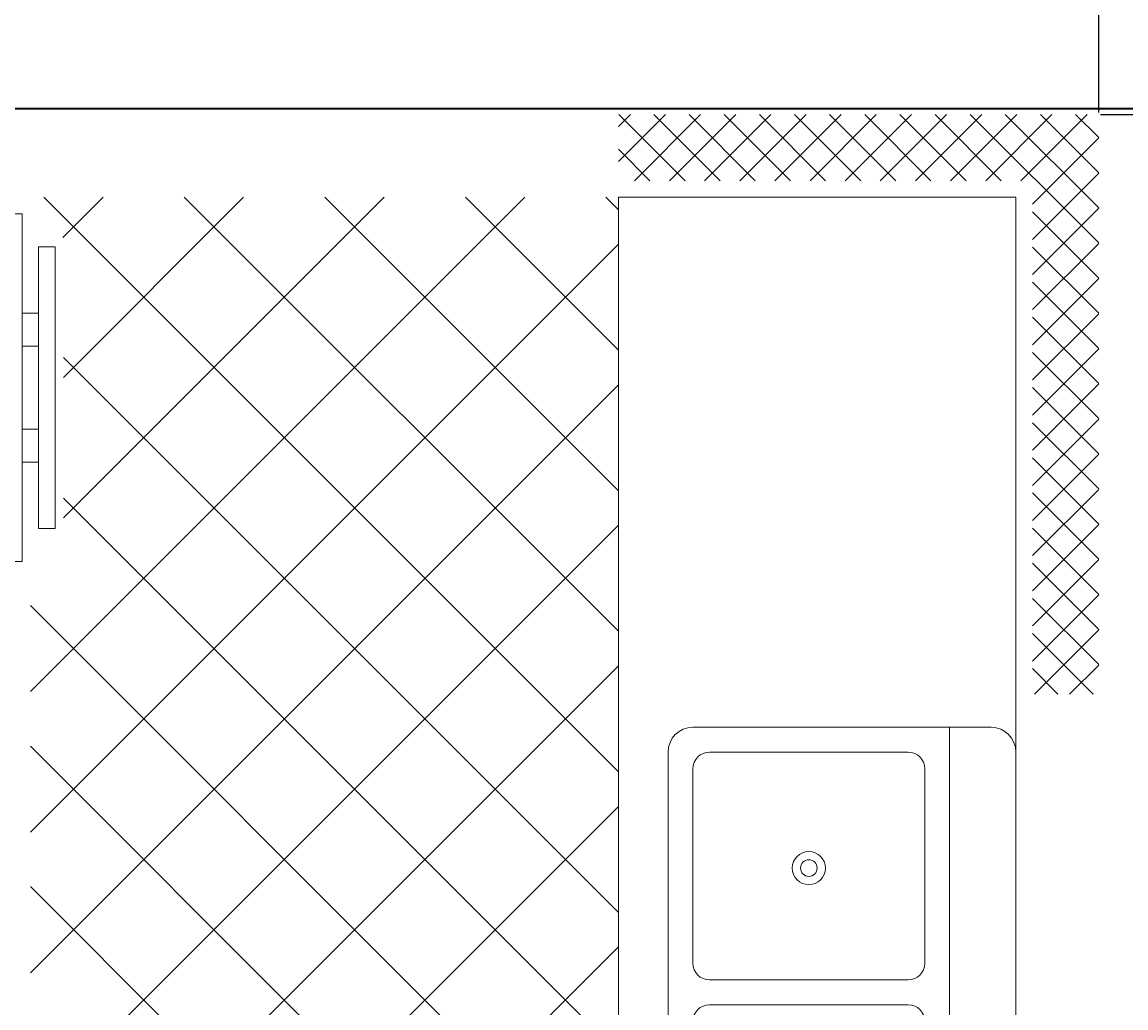
# Model space of a CAD drawing. Units: inches. Extents: x 4159 to 4826, y 299 to 1026.
# Tile 16 of 37: x 4218 to 4255, y 630 to 663. Entities that reach past the tile are written whole.
import ezdxf

# ---------------------------------------------------------------- set-up
doc = ezdxf.new("R2010")
doc.units = ezdxf.units.IN
for name, color, linetype, lineweight in [('A-ANNO-DIMS', 2, 'Continuous', 18), ('A-FLOR-FIXT', 9, 'Continuous', 18), ('A-WALL', 7, 'Continuous', 35)]:
    doc.layers.add(name, color=color, linetype=linetype, lineweight=lineweight)
doc.styles.get("Standard").update_dxf_attribs({"font": 'arial.ttf'})
doc.dimstyles.get("Standard").update_dxf_attribs({"dimtxt": 0.18, "dimasz": 0.18, "dimexe": 0.18, "dimexo": 0.0625, "dimgap": 0.09, "dimtad": 0, "dimtih": 1, "dimtoh": 1, "dimdec": 4, "dimzin": 0, "dimdsep": 46, "dimtxsty": 'Standard', "dimcen": 0.09, "dimadec": 0, "dimazin": 0, "dimtfac": 1, "dimtdec": 4, "dimtofl": 0, "dimtmove": 0, "dimatfit": 3, "dimfxl": 1, "dimtolj": 1, "dimtzin": 0, "dimarcsym": 0})

# ---------------------------------------------------------------- blocks, each defined once
blk = doc.blocks.new('Kitchen Layout - 7 x 8 ft')
for p, q in [((80, 60), (80, 59)), ((82, 59), (82, 60)), ((87, 59), (87, 60)), ((89, 60), (89, 59)), ((18.882, 24), (54.382, 59.5)), ((27.368, 24), (62.868, 59.5)), ((35.853, 24), (71.353, 59.5)), ((76.199, 24), (40.699, 59.5)), ((84.684, 24), (49.184, 59.5)), ((93.169, 24), (57.669, 59.5)), ((96, 29.655), (66.155, 59.5)), ((61.309, 24), (96, 58.691)), ((67.714, 24), (33.675, 58.038)), ((44.338, 24), (77.838, 57.5)), ((52.823, 24), (86.323, 57.5)), ((96, 38.14), (76.64, 57.5)), ((96, 46.625), (85.125, 57.5)), ((96, 55.111), (93.569, 57.541)), ((50.743, 24), (19.743, 55)), ((59.228, 24), (28.228, 55)), ((69.794, 24), (96, 50.206)), ((78.279, 24), (96, 41.721)), ((86.764, 24), (96, 33.236)), ((95.25, 24), (96, 24.75)), ((0, 24), (96, 24)), ((96, 24), (96, 0)), ((97, 22.095), (98.905, 24)), ((101, 21.155), (98.155, 24)), ((101, 23.276), (100.276, 24)), ((97, 19.974), (101, 23.974)), ((101, 19.034), (97, 23.034)), ((97, 17.853), (101, 21.853)), ((101, 16.913), (97, 20.913)), ((97, 15.731), (101, 19.731)), ((101, 14.791), (97, 18.791)), ((47.25, 6.5), (47.25, 18.5)), ((48.75, 18.5), (48.75, 6.5)), ((97, 13.61), (101, 17.61)), ((101, 12.67), (97, 16.67)), ((97, 11.489), (101, 15.489)), ((101, 10.549), (97, 14.549)), ((97, 9.367), (101, 13.367)), ((101, 8.427), (97, 12.427)), ((97, 7.246), (101, 11.246)), ((101, 6.306), (97, 10.306)), ((97, 5.125), (101, 9.125)), ((101, 4.185), (97, 8.185)), ((97, 3.003), (101, 7.003)), ((101, 2.063), (97, 6.063)), ((97, 0.882), (101, 4.882)), ((64, 4), (32, 4)), ((101, -0.058), (97, 3.942)), ((93.239, -5), (101, 2.761)), ((101, -2.179), (97, 1.821)), ((96, 0), (0, 0)), ((95.361, -5), (101, 0.639)), ((101, -4.301), (97, -0.301)), ((66, -2.541), (67.541, -1)), ((66, -4.662), (69.662, -1)), ((69.88, -5), (66, -1.12)), ((67.783, -5), (71.783, -1)), ((72.001, -5), (68.001, -1)), ((69.905, -5), (73.905, -1)), ((74.122, -5), (70.122, -1)), ((72.026, -5), (76.026, -1)), ((76.243, -5), (72.243, -1)), ((74.147, -5), (78.147, -1)), ((78.365, -5), (74.365, -1)), ((76.269, -5), (80.269, -1)), ((80.486, -5), (76.486, -1)), ((78.39, -5), (82.39, -1)), ((82.607, -5), (78.607, -1)), ((80.511, -5), (84.511, -1)), ((84.729, -5), (80.729, -1)), ((82.633, -5), (86.633, -1)), ((86.85, -5), (82.85, -1)), ((84.754, -5), (88.754, -1)), ((88.971, -5), (84.971, -1)), ((86.875, -5), (90.875, -1)), ((91.093, -5), (87.093, -1)), ((88.997, -5), (92.997, -1)), ((93.214, -5), (89.214, -1)), ((91.118, -5), (95.118, -1)), ((95.335, -5), (91.335, -1)), ((97.457, -5), (93.457, -1)), ((99.578, -5), (95.578, -1)), ((97.482, -5), (101, -1.482)), ((67.758, -5), (66, -3.242)), ((99.603, -5), (101, -3.603))]:
    blk.add_line(p, q)
for points in [[(74, 60), (74, 84), (95, 84), (95, 60)], [(76, 58), (76, 59), (93, 59), (93, 58)]]:
    blk.add_lwpolyline(points, close=True)
for points in [[(33.5, 21), (62.5, 21)], [(49.75, 19.5), (61.5, 19.5)], [(64, 19.5), (64, 1.5)], [(62.5, 18.5), (62.5, 6.5)], [(61.5, 5.5), (49.75, 5.5)], [(62.5, 0), (33.5, 0)]]:
    blk.add_lwpolyline(points)
for radius in [1, 0.5]:
    blk.add_circle((55.5, 12.5), radius)
for centre, radius, start, end in [((62.5, 19.5), 1.5, 0, 90), ((46.25, 18.5), 1, 0, 90), ((49.75, 18.5), 1, 90, 180), ((61.5, 18.5), 1, 0, 90), ((46.25, 6.5), 1, 270, 0), ((49.75, 6.5), 1, 180, 270), ((61.5, 6.5), 1, 270, 0), ((62.5, 1.5), 1.5, 270, 0)]:
    blk.add_arc(centre, radius, start, end)
blk = doc.blocks.new('*D39')
at = {"layer": 'A-ANNO-DIMS', "color": 0, "lineweight": -2, "transparency": 16777216}
for p, q in [((4254.612, 660.06), (4263.714, 660.06)), ((4263.534, 659.88), (4263.534, 630.296)), ((4263.534, 600.346), (4263.534, 629.93)), ((4254.612, 600.166), (4263.714, 600.166))]:
    blk.add_line(p, q, dxfattribs=at)
at = {"layer": 'A-ANNO-DIMS', "color": 0, "transparency": 16777216}
for points in [[(4263.504, 659.88), (4263.564, 659.88), (4263.534, 660.06)], [(4263.504, 600.346), (4263.564, 600.346), (4263.534, 600.166)]]:
    blk.add_solid(points, dxfattribs=at)
at = {"layer": 'Defpoints', "color": 0, "transparency": 16777216}
for p in [(4254.55, 660.06), (4263.534, 660.06), (4254.55, 600.166)]:
    blk.add_point(p, dxfattribs=at)
at = {"layer": 'A-ANNO-DIMS', "color": 0, "transparency": 16777216, "insert": (4263.534, 630.113), "char_height": 0.18, "attachment_point": 5}
blk.add_mtext('\\A1;KITCHEN 60 TYP.', dxfattribs=at)
blk = doc.blocks.new('*D40')
at = {"layer": 'A-ANNO-DIMS', "color": 0, "lineweight": -2, "transparency": 16777216}
for p, q in [((4201.437, 660.122), (4201.437, 669.224)), ((4254.55, 660.122), (4254.55, 669.224)), ((4201.617, 669.044), (4227.465, 669.044)), ((4254.37, 669.044), (4228.521, 669.044))]:
    blk.add_line(p, q, dxfattribs=at)
at = {"layer": 'A-ANNO-DIMS', "color": 0, "transparency": 16777216}
for points in [[(4201.617, 669.074), (4201.617, 669.014), (4201.437, 669.044)], [(4254.37, 669.074), (4254.37, 669.014), (4254.55, 669.044)]]:
    blk.add_solid(points, dxfattribs=at)
at = {"layer": 'Defpoints', "color": 0, "transparency": 16777216}
for p in [(4201.437, 669.044), (4201.437, 660.06), (4254.55, 660.06)]:
    blk.add_point(p, dxfattribs=at)
at = {"layer": 'A-ANNO-DIMS', "color": 0, "transparency": 16777216, "insert": (4227.993, 669.044), "char_height": 0.18, "attachment_point": 5}
blk.add_mtext('\\A1;53 TYP.', dxfattribs=at)
blk = doc.blocks.new('*D44')
at = {"layer": 'A-ANNO-DIMS', "color": 0, "lineweight": -2, "transparency": 16777216}
for p, q in [((4287.263, 963.093), (4158.88, 963.093)), ((4159.06, 962.913), (4159.06, 647.826)), ((4159.06, 332.375), (4159.06, 647.462)), ((4447.248, 332.195), (4158.88, 332.195))]:
    blk.add_line(p, q, dxfattribs=at)
at = {"layer": 'A-ANNO-DIMS', "color": 0, "transparency": 16777216}
for points in [[(4159.03, 962.913), (4159.09, 962.913), (4159.06, 963.093)], [(4159.03, 332.375), (4159.09, 332.375), (4159.06, 332.195)]]:
    blk.add_solid(points, dxfattribs=at)
at = {"layer": 'Defpoints', "color": 0, "transparency": 16777216}
for p in [(4287.326, 963.093), (4159.06, 332.195), (4447.31, 332.195)]:
    blk.add_point(p, dxfattribs=at)
at = {"layer": 'A-ANNO-DIMS', "color": 0, "transparency": 16777216, "insert": (4159.06, 647.644), "char_height": 0.18, "attachment_point": 5}
blk.add_mtext('\\A1;630.9', dxfattribs=at)

msp = doc.modelspace()

# ---------------------------------------------------------------- linework, layer by layer
at = {"layer": 'A-WALL'}
msp.add_line((4447.31, 660.254), (4201.31, 660.254), dxfattribs=at)

# ---------------------------------------------------------------- block references
at = {"layer": 'A-FLOR-FIXT', "xscale": 0.5650329326971529, "yscale": 0.5650329326971529, "zscale": 0.5650329326971529, "rotation": 90}
msp.add_blockref('Kitchen Layout - 7 x 8 ft', (4251.725, 602.991), dxfattribs=at)

# ---------------------------------------------------------------- dimensions: what is measured, and where the dimension line sits
at = {"layer": 'A-ANNO-DIMS'}
dim = msp.add_linear_dim(base=(4159.06, 332.195), p1=(4287.326, 963.093), p2=(4447.31, 332.195), angle=90, dimstyle='Standard', override={"dimdec": 1, "dimlfac": 1, "dimrnd": 0, "dimzin": 0, "dimdsep": 46, "dimlunit": 2}, dxfattribs=at)
dim.commit()
dim.dimension.update_dxf_attribs({"geometry": '*D44', "text_midpoint": (4159.06, 647.644)})
for base, p1, p2, angle, text, picture, middle in [((4201.437, 669.044), (4254.55, 660.06), (4201.437, 660.06), 180, '<> TYP.', '*D40', (4227.993, 669.044)), ((4263.534, 660.06), (4254.55, 600.166), (4254.55, 660.06), 90, 'KITCHEN <> TYP.', '*D39', (4263.534, 630.113))]:
    dim = msp.add_linear_dim(base=base, p1=p1, p2=p2, angle=angle, text=text, dimstyle='Standard', override={"dimdec": 0, "dimlfac": 1, "dimrnd": 0, "dimzin": 0, "dimdsep": 46, "dimlunit": 2}, dxfattribs=at)
    dim.commit()
    dim.dimension.update_dxf_attribs({"geometry": picture, "text_midpoint": middle})

doc.saveas('drawing.dxf')
